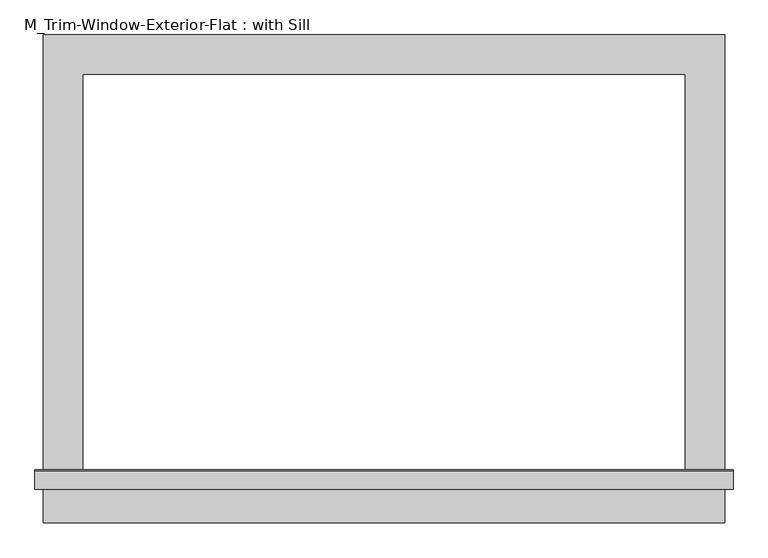
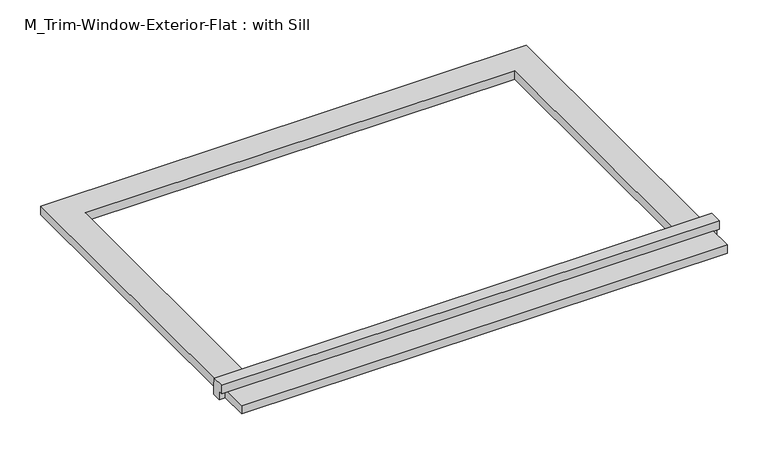
"""IFC4 building model written with IfcOpenShell, lengths in millimetres: proxy geometry, M_Trim-Window-Exterior-Flat : with Sill."""

from ifc_helpers import new_model, si_unit, frame, origin, origin_with_axes, place, context, project, spatial, polyline, outline, extrude, source, transform, mapped, element, save


def m_trim_window_exterior_flat_with_sill_78b3ef69(model_context):
    return source(origin(), model_context, "Body", "SweptSolid", [
        extrude(outline(polyline([(517.2, -620.4323709), (517.2, -680.4323709), (-517.2, -680.4323709), (-517.2, -620.4323709), (517.2, -620.4323709)])), origin_with_axes(), (0.0, 0.0, 1.0), 19.05),
        extrude(outline(polyline([(-630.0, 38.1), (-602.4580645, 38.1), (-600.0, 19.05), (-600.0, 0.0), (-620.4323709, 0.0), (-620.4323709, 19.05), (-630.0, 19.05), (-630.0, 38.1)])), frame((-529.9, 0.0, 0.0), z_axis=(1.0, 0.0, 0.0), x_axis=(0.0, 1.0, 0.0)), (0.0, 0.0, 1.0), 1059.8),
        extrude(outline(polyline([(-517.2, 60.0), (517.2, 60.0), (517.2, -600.0), (457.2, -600.0), (457.2, 0.0), (-457.2, 0.0), (-457.2, -600.0), (-517.2, -600.0), (-517.2, 60.0)])), origin_with_axes(), (0.0, 0.0, 1.0), 19.05),
    ])


if __name__ == "__main__":
    model = new_model("IFC4")
    model_context = context("Model", 3, world=origin())
    ifc_project = project(units=[si_unit("LENGTHUNIT", "METRE", prefix="MILLI")], contexts=[model_context])
    site = spatial("IfcSite", under=ifc_project)
    building = spatial("IfcBuilding", under=site)
    placement = place(None, origin())
    m_trim_window_exterior_flat_with_sill_shape = m_trim_window_exterior_flat_with_sill_78b3ef69(model_context)
    element("IfcBuildingElementProxy", 1, Name="M_Trim-Window-Exterior-Flat : with Sill", ObjectType="M_Trim-Window-Exterior-Flat : with Sill", at=placement, inside=building, context=model_context, shape_type="MappedRepresentation", body=[
        mapped(m_trim_window_exterior_flat_with_sill_shape, transform((0.0, 0.0, 0.0), x_axis=(1.0, 0.0, 0.0), y_axis=(0.0, 1.0, 0.0), z_axis=(0.0, 0.0, 1.0))),
    ])
    save(model, "model.ifc")

# Revit data of these elements
# Type "M_Trim-Window-Exterior-Flat : with Sill"
#   Trim Width = 0' - 2.3622"
#   Trim Thickness_Picture Frame = 0' - 1.1811"
#   Trim Thickness_with Sill = 0' - 0 3/4"
#   Sill Thickness = 0' - 1.1811"
#   Opening Width [instance default] = 1' - 11.62205"
#   Opening Height [instance default] = 2' - 11.43307"
#   Default Elevation = 3' - 11.24409"
#   Sill = yes
#   Picture Frame = no
#   Trim Material [instance default] = none
# Element 1 (IfcBuildingElementProxy, "M_Trim-Window-Exterior-Flat : with Sill")
#   Opening Width = 3' - 0"
#   Opening Height = 1' - 11.62205"
#   Trim Material = Clad - White
#   Materials on its faces: "Clad - White"
# Materials
#   "Clad - White": class "Wood", colour RGB 242 242 238, transparency 0, Cost = 0
